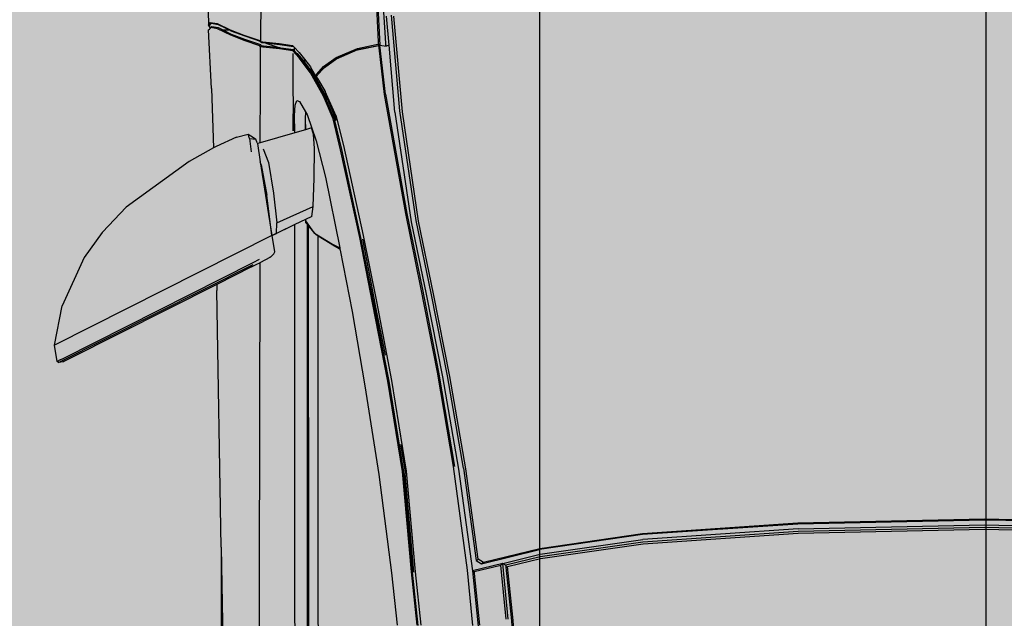
# Model space of a CAD drawing. Units: inches. Extents: x 1884 to 2398, y 474 to 1488.
# Tile 11 of 39: x 2186 to 2231, y 672 to 699. Entities that reach past the tile are written whole.
import ezdxf

# ---------------------------------------------------------------- set-up
doc = ezdxf.new("R2010")
doc.units = ezdxf.units.IN
doc.header["$MEASUREMENT"] = 0
doc.layers.get('0').update_dxf_attribs({"color": 250})
doc.layers.add('A-ANNO-DIMS', color=2, linetype='Continuous', lineweight=18)
doc.layers.add('C-VEHI', color=8, linetype='Continuous', lineweight=18)
doc.layers.add('Edges', color=250, linetype='Continuous')
doc.layers.add('L-PVMT-PATT', color=9, linetype='Continuous', lineweight=13, true_color=0xc7c8ca)
doc.styles.get("Standard").update_dxf_attribs({"font": 'arial.ttf'})
doc.dimstyles.get("Standard").update_dxf_attribs({"dimtxt": 7, "dimasz": 0.18, "dimexe": 0.18, "dimexo": 0.0625, "dimgap": 0.09, "dimtad": 0, "dimtih": 1, "dimtoh": 1, "dimzin": 0, "dimdsep": 46, "dimlunit": 3, "dimtxsty": 'Standard', "dimcen": 0.09, "dimadec": 0, "dimazin": 0, "dimtfac": 1, "dimtofl": 0, "dimtmove": 0, "dimatfit": 3, "dimfxl": 1, "dimtolj": 1, "dimtzin": 0, "dimarcsym": 0})

# ---------------------------------------------------------------- blocks, each defined once
blk = doc.blocks.new('Nissan Qashqai pl')
at = {"layer": 'Edges'}
for p, q in [((9.2241, 12.1376), (9.2195, 11.9221)), ((9.2249, 12.1376), (9.2203, 11.9221)), ((9.2259, 11.9221), (9.2305, 12.1375)), ((9.2335, 12.1374), (9.2289, 11.9221)), ((9.2308, 11.9221), (9.2355, 12.1374)), ((9.2195, 11.9221), (9.2241, 11.7066)), ((9.2203, 11.9221), (9.2249, 11.7065)), ((9.2305, 11.7067), (9.2259, 11.9221)), ((9.2289, 11.9221), (9.2335, 11.7067)), ((9.2355, 11.7068), (9.2308, 11.9221)), ((9.2241, 11.7066), (9.2362, 11.5274)), ((9.2249, 11.7065), (9.2371, 11.5273)), ((9.2305, 11.7067), (9.2426, 11.5277)), ((9.2335, 11.7067), (9.2457, 11.5277)), ((9.2476, 11.5278), (9.2355, 11.7068)), ((9.2362, 11.5274), (9.2535, 11.4087)), ((9.2371, 11.5273), (9.2543, 11.4085)), ((9.2598, 11.4093), (9.2426, 11.5277)), ((9.2457, 11.5277), (9.2629, 11.4092)), ((9.2649, 11.4094), (9.2476, 11.5278)), ((9.2535, 11.4087), (9.2694, 11.3436)), ((9.2707, 11.3414), (9.2543, 11.4085)), ((9.2704, 11.3659), (9.2598, 11.4093)), ((9.2629, 11.4092), (9.2726, 11.3695)), ((9.2741, 11.3716), (9.2649, 11.4094)), ((9.3326, 11.3776), (9.2741, 11.3716)), ((9.2746, 11.3697), (9.333, 11.3757)), ((9.4, 11.3832), (9.3326, 11.3776)), ((9.333, 11.3757), (9.4004, 11.3813)), ((9.3346, 11.3724), (9.2704, 11.3659)), ((9.2704, 11.3659), (9.2726, 11.3695)), ((9.2704, 11.3659), (9.2724, 11.3637)), ((9.2704, 11.3659), (9.2789, 11.331)), ((9.3346, 11.37), (9.2724, 11.3637)), ((9.2799, 11.3328), (9.2724, 11.3637)), ((9.2726, 11.3695), (9.2746, 11.3697)), ((9.2694, 11.3436), (9.2656, 11.3376)), ((9.2669, 11.3354), (9.2707, 11.3414)), ((9.2694, 11.3436), (9.2707, 11.3414)), ((9.2819, 11.333), (9.3418, 11.3391)), ((9.1605, 11.3208), (9.2669, 11.3354)), ((9.2656, 11.3376), (9.1612, 11.3233)), ((9.1617, 11.315), (9.2789, 11.331)), ((9.2669, 11.3354), (9.2656, 11.3376)), ((9.3422, 11.3316), (9.2783, 11.3251)), ((9.2789, 11.331), (9.3427, 11.3375)), ((9.2789, 11.331), (9.2799, 11.3327)), ((9.2799, 11.3328), (9.2819, 11.333)), ((9.2799, 11.3327), (9.2799, 11.3328)), ((9.2799, 11.3327), (9.2811, 11.3325)), ((9.1605, 11.3208), (9.0538, 11.3023)), ((9.1612, 11.3233), (9.0546, 11.3048)), ((9.2783, 11.3251), (9.1584, 11.3091)), ((9.0546, 11.3048), (8.9591, 11.2859)), ((9.1584, 11.3091), (9.0495, 11.2906)), ((9.0497, 11.2918), (9.1586, 11.3104)), ((9.0552, 11.2965), (9.1617, 11.315)), ((9.0538, 11.3023), (8.9583, 11.2833)), ((8.9598, 11.2775), (9.0552, 11.2965)), ((8.9583, 11.2833), (8.8745, 11.266)), ((8.9591, 11.2859), (8.8754, 11.2687)), ((9.0495, 11.2906), (8.9521, 11.2715)), ((8.9522, 11.2728), (9.0497, 11.2918)), ((8.8666, 11.2554), (8.9522, 11.2728)), ((8.9521, 11.2715), (8.8666, 11.2541)), ((8.8761, 11.2602), (8.9598, 11.2775)), ((9.2801, 11.2648), (9.3418, 11.2713)), ((8.8745, 11.266), (8.7481, 11.2473)), ((8.8754, 11.2687), (8.7491, 11.2501)), ((8.7496, 11.2416), (8.8761, 11.2602)), ((9.1639, 11.2546), (9.2801, 11.2648)), ((9.2803, 11.2606), (9.1644, 11.2503)), ((9.2804, 11.262), (9.1645, 11.2518)), ((9.2804, 11.2635), (9.1668, 11.2533)), ((9.3418, 11.2671), (9.2803, 11.2606)), ((9.3419, 11.2685), (9.2804, 11.262)), ((8.7491, 11.2501), (8.6386, 11.2404)), ((8.7287, 11.2307), (8.8666, 11.2554)), ((8.8666, 11.2541), (8.7292, 11.2295)), ((9.0591, 11.2377), (9.1639, 11.2546)), ((9.1644, 11.2503), (9.06, 11.2335)), ((9.1645, 11.2518), (9.0601, 11.235)), ((9.133, 11.2481), (9.1647, 11.2532)), ((9.1647, 11.2532), (9.1668, 11.2533)), ((8.7481, 11.2473), (8.6375, 11.2376)), ((8.7496, 11.2416), (8.6721, 11.2348)), ((8.9679, 11.2201), (9.0591, 11.2377)), ((9.1676, 11.2229), (9.2814, 11.2377)), ((9.2814, 11.2377), (9.3416, 11.2442)), ((8.6699, 11.231), (8.622, 11.228)), ((8.6721, 11.2348), (8.6387, 11.2319)), ((8.6721, 11.2312), (8.6699, 11.231)), ((8.6721, 11.2348), (8.6733, 11.2313)), ((8.6721, 11.2312), (8.6721, 11.2318)), ((8.6721, 11.2241), (8.6733, 11.2313)), ((8.6733, 11.2313), (8.6721, 11.2312)), ((8.7287, 11.2307), (8.6721, 11.2241)), ((8.7292, 11.2295), (8.6753, 11.2232)), ((9.0601, 11.235), (8.8941, 11.2023)), ((9.06, 11.2335), (8.9696, 11.2157)), ((8.9708, 11.2185), (9.03, 11.2304)), ((8.6683, 11.2226), (8.6197, 11.2201)), ((8.6203, 11.2213), (8.6721, 11.2241)), ((8.671, 11.2227), (8.6683, 11.2226)), ((8.6721, 11.2241), (8.671, 11.2227)), ((8.6716, 11.2199), (8.671, 11.2227)), ((8.6759, 11.1982), (8.6716, 11.2199)), ((8.6721, 11.2241), (8.6727, 11.2229)), ((8.6772, 11.1988), (8.6721, 11.2241)), ((8.6753, 11.2232), (8.6727, 11.2229)), ((8.6777, 11.1984), (8.6727, 11.2229)), ((8.8918, 11.205), (8.9679, 11.2201)), ((8.9696, 11.2157), (8.8942, 11.2009)), ((8.9318, 11.211), (8.9704, 11.2185)), ((8.9704, 11.2185), (8.9708, 11.2185)), ((9.0656, 11.207), (9.1676, 11.2229)), ((8.7881, 11.1821), (8.8918, 11.205)), ((8.8941, 11.2023), (8.7925, 11.1802)), ((8.8961, 11.204), (8.9318, 11.211)), ((8.9797, 11.1924), (9.0656, 11.207)), ((8.6864, 11.1736), (8.6759, 11.1982)), ((8.6875, 11.1744), (8.6772, 11.1988)), ((8.6777, 11.1984), (8.6883, 11.1737)), ((8.8942, 11.2009), (8.7931, 11.1789)), ((8.9087, 11.1783), (8.9797, 11.1924)), ((8.7575, 11.1744), (8.7881, 11.1821)), ((8.7925, 11.1802), (8.7591, 11.1723)), ((8.697, 11.1592), (8.6864, 11.1736)), ((8.6979, 11.1603), (8.6875, 11.1744)), ((8.6883, 11.1737), (8.6987, 11.1597)), ((8.7508, 11.1722), (8.7257, 11.1609)), ((8.7529, 11.17), (8.7302, 11.1602)), ((8.7574, 11.1704), (8.7312, 11.1591)), ((8.7346, 11.1636), (8.7577, 11.1732)), ((8.7346, 11.1636), (8.7491, 11.1703)), ((8.7491, 11.1703), (8.7576, 11.1743)), ((8.7508, 11.1722), (8.7491, 11.1703)), ((8.7532, 11.1733), (8.7508, 11.1722)), ((8.7529, 11.17), (8.7577, 11.1732)), ((8.757, 11.1718), (8.7529, 11.17)), ((8.7532, 11.1733), (8.7575, 11.1744)), ((8.7587, 11.1722), (8.757, 11.1718)), ((8.7931, 11.1789), (8.7574, 11.1704)), ((8.7575, 11.1744), (8.7576, 11.1743)), ((8.7576, 11.1743), (8.7582, 11.1734)), ((8.7577, 11.1732), (8.7582, 11.1734)), ((8.7582, 11.1734), (8.759, 11.1725)), ((8.759, 11.1725), (8.7587, 11.1722)), ((8.7591, 11.1723), (8.7587, 11.1722)), ((8.759, 11.1725), (8.7591, 11.1723)), ((8.8245, 11.1613), (8.9063, 11.1779)), ((8.8893, 11.1486), (8.9021, 11.1697)), ((8.9041, 11.1717), (8.8927, 11.1528)), ((8.9021, 11.1697), (8.9063, 11.1779)), ((8.9075, 11.1781), (8.9041, 11.1717)), ((8.9063, 11.1779), (8.9075, 11.1781)), ((8.9075, 11.1781), (8.9087, 11.1783)), ((8.7055, 11.1514), (8.697, 11.1592)), ((8.6987, 11.1596), (8.6979, 11.1603)), ((8.6987, 11.1597), (8.6988, 11.1596)), ((8.6987, 11.1596), (8.6988, 11.1596)), ((8.6996, 11.1588), (8.6987, 11.1596)), ((8.6988, 11.1596), (8.6996, 11.1588)), ((8.6996, 11.1588), (8.6996, 11.1588)), ((8.7062, 11.1527), (8.6996, 11.1588)), ((8.6996, 11.1588), (8.7062, 11.1527)), ((8.7302, 11.1602), (8.7032, 11.145)), ((8.7312, 11.1591), (8.7042, 11.144)), ((8.7075, 11.1487), (8.7346, 11.1636)), ((8.7108, 11.1523), (8.7257, 11.1609)), ((8.7108, 11.1523), (8.7248, 11.1605)), ((8.7248, 11.1605), (8.7257, 11.1609)), ((8.7828, 11.1508), (8.8245, 11.1613)), ((8.6917, 11.1371), (8.7075, 11.1487)), ((8.7071, 11.15), (8.6981, 11.1446)), ((8.707, 11.15), (8.7055, 11.1514)), ((8.7067, 11.1522), (8.7062, 11.1527)), ((8.7083, 11.1508), (8.7067, 11.1522)), ((8.707, 11.15), (8.7083, 11.1508)), ((8.7071, 11.15), (8.707, 11.15)), ((8.707, 11.15), (8.707, 11.15)), ((8.7083, 11.1508), (8.7071, 11.15)), ((8.7083, 11.1507), (8.7102, 11.1519)), ((8.7083, 11.1508), (8.7083, 11.1507)), ((8.7102, 11.1519), (8.7108, 11.1523)), ((8.7524, 11.1401), (8.7828, 11.1508)), ((8.7748, 11.1475), (8.7678, 11.1453)), ((8.7678, 11.1453), (8.7698, 11.1385)), ((8.7916, 11.1488), (8.7748, 11.1475)), ((8.8259, 11.1483), (8.7916, 11.1488)), ((8.8585, 11.1473), (8.8259, 11.1483)), ((8.87, 11.1455), (8.8585, 11.1473)), ((8.8771, 11.1054), (8.8585, 11.1473)), ((8.87, 11.1455), (8.8734, 11.1385)), ((8.8893, 11.1486), (8.8751, 11.1387)), ((8.881, 11.1418), (8.8893, 11.1486)), ((8.8913, 11.1506), (8.8893, 11.1486)), ((8.8927, 11.1528), (8.8913, 11.1506)), ((9.3225, 11.1531), (8.8927, 11.1528)), ((9.4936, 11.1538), (9.3225, 11.1531)), ((8.6805, 11.1309), (8.6884, 11.1371)), ((8.6818, 11.1288), (8.6902, 11.136)), ((8.6927, 11.1371), (8.6859, 11.132)), ((8.7042, 11.144), (8.687, 11.131)), ((8.6884, 11.1371), (8.6973, 11.144)), ((8.6884, 11.1371), (8.6917, 11.1371)), ((8.6902, 11.136), (8.6917, 11.1371)), ((8.6923, 11.1371), (8.6927, 11.1371)), ((8.7032, 11.145), (8.6927, 11.1371)), ((8.6973, 11.144), (8.698, 11.1446)), ((8.698, 11.1446), (8.6981, 11.1446)), ((8.7373, 11.1314), (8.7492, 11.1383)), ((8.7492, 11.1383), (8.7524, 11.1401)), ((8.7492, 11.1383), (8.7572, 11.1379)), ((8.7572, 11.1379), (8.7698, 11.1383)), ((8.7698, 11.1385), (8.7583, 11.1382)), ((8.7698, 11.1385), (8.7698, 11.1383)), ((8.7698, 11.1383), (8.7733, 11.126)), ((8.8734, 11.1385), (8.8793, 11.1261)), ((8.8734, 11.1385), (8.8768, 11.1385)), ((8.8751, 11.1387), (8.8768, 11.1385)), ((8.8768, 11.1385), (8.879, 11.1402)), ((8.879, 11.1402), (8.881, 11.1418)), ((8.879, 11.1402), (9.3198, 11.1403)), ((9.3225, 11.1421), (8.881, 11.1418)), ((9.3198, 11.1403), (9.4922, 11.1409)), ((9.4936, 11.1428), (9.3225, 11.1421)), ((8.6703, 11.1081), (8.6727, 11.1235)), ((8.6714, 11.1088), (8.6737, 11.1245)), ((8.6727, 11.1235), (8.6737, 11.1245)), ((8.6737, 11.1245), (8.6746, 11.1253)), ((8.6805, 11.1309), (8.6746, 11.1253)), ((8.6746, 11.1253), (8.6785, 11.1253)), ((8.6777, 11.1246), (8.6755, 11.1099)), ((8.6788, 11.1237), (8.6764, 11.1083)), ((8.6785, 11.1253), (8.6777, 11.1246)), ((8.6815, 11.128), (8.6785, 11.1253)), ((8.687, 11.131), (8.6788, 11.1237)), ((8.6815, 11.128), (8.6818, 11.1288)), ((8.6817, 11.1282), (8.6815, 11.128)), ((8.6859, 11.132), (8.6817, 11.1282)), ((8.6817, 11.1282), (8.6818, 11.1288)), ((8.6818, 11.1238), (8.7026, 11.1238)), ((8.7026, 11.1238), (8.7026, 11.1239)), ((8.7026, 11.1238), (8.7072, 11.1239)), ((8.7072, 11.1239), (8.7072, 11.1239)), ((8.7072, 11.1239), (8.7273, 11.1239)), ((8.7273, 11.1239), (8.7273, 11.124)), ((8.7273, 11.1239), (8.7354, 11.124)), ((8.7354, 11.1241), (8.7354, 11.124)), ((8.7354, 11.124), (8.742, 11.124)), ((8.7361, 11.1283), (8.7373, 11.1314)), ((8.7415, 11.1265), (8.7361, 11.1283)), ((8.7534, 11.1257), (8.7415, 11.1265)), ((8.742, 11.1241), (8.742, 11.124)), ((8.742, 11.124), (8.742, 11.1241)), ((8.742, 11.124), (8.742, 11.124)), ((8.742, 11.124), (8.7426, 11.124)), ((8.7426, 11.1241), (8.7426, 11.124)), ((8.7426, 11.124), (8.7433, 11.124)), ((8.7433, 11.1241), (8.7433, 11.124)), ((8.7433, 11.124), (8.7711, 11.1241)), ((8.7711, 11.1241), (8.7516, 11.1241)), ((8.7718, 11.126), (8.7534, 11.1257)), ((8.7733, 11.126), (8.7718, 11.126)), ((8.7733, 11.126), (8.7849, 11.0859)), ((9.3194, 11.1262), (8.8793, 11.1261)), ((8.8793, 11.1261), (8.8815, 11.1214)), ((9.4919, 11.1269), (9.3194, 11.1262)), ((8.8815, 11.1214), (8.892, 11.0998)), ((8.8815, 11.1214), (8.8895, 11.1048)), ((8.6684, 11.0892), (8.6703, 11.1081)), ((8.6697, 11.0922), (8.6714, 11.1088)), ((8.6698, 11.0925), (8.6755, 11.1099)), ((8.6754, 11.1089), (8.6735, 11.0898)), ((8.6764, 11.1082), (8.6744, 11.0891)), ((8.6755, 11.1099), (8.6754, 11.1089)), ((8.6764, 11.1082), (8.6764, 11.1083)), ((8.807, 11.0862), (8.8918, 11.0997)), ((8.8075, 11.0955), (8.8429, 11.1016)), ((8.8429, 11.1016), (8.8771, 11.1054)), ((8.8918, 11.0997), (8.8455, 11.0936)), ((8.8895, 11.1048), (8.8771, 11.1054)), ((8.8908, 11.1021), (8.8895, 11.1048)), ((8.8906, 11.1024), (8.8895, 11.1048)), ((8.8906, 11.1024), (8.8911, 11.1013)), ((8.892, 11.0998), (8.8908, 11.1021)), ((8.8911, 11.1013), (8.8919, 11.0997)), ((8.8911, 11.1013), (8.8919, 11.0998)), ((8.8919, 11.0997), (8.8911, 11.1013)), ((8.8919, 11.0997), (8.8918, 11.0997)), ((8.8918, 11.0997), (9.0186, 10.8486)), ((8.892, 11.0998), (8.8919, 11.0998)), ((8.8919, 11.0998), (8.8919, 11.0997)), ((8.8919, 11.0997), (8.8919, 11.0997)), ((8.9106, 11.1029), (8.892, 11.0998)), ((8.892, 11.0998), (8.892, 11.0998)), ((8.9131, 11.102), (8.9106, 11.1029)), ((8.9171, 11.0978), (8.9131, 11.102)), ((8.6682, 11.087), (8.6684, 11.0888)), ((8.6684, 11.0888), (8.6684, 11.0892)), ((8.6684, 11.0888), (8.6685, 11.089)), ((8.6692, 11.0876), (8.6697, 11.0922)), ((8.6697, 11.0922), (8.6698, 11.0925)), ((8.6735, 11.0898), (8.6733, 11.0875)), ((8.6744, 11.0891), (8.6742, 11.0866)), ((8.7917, 11.0895), (8.8075, 11.0955)), ((8.8102, 11.0874), (8.8455, 11.0936)), ((8.9171, 11.0978), (8.917, 11.0974)), ((8.9171, 11.0978), (8.9233, 11.0855)), ((8.5326, 11.0874), (8.6675, 11.0866)), ((8.6606, 11.0674), (8.6667, 11.0857)), ((8.6616, 11.0683), (8.6675, 11.0862)), ((8.6718, 11.0868), (8.6657, 11.0684)), ((8.6667, 11.0857), (8.6675, 11.0862)), ((8.6728, 11.0858), (8.6667, 11.0675)), ((8.6674, 11.0864), (8.6675, 11.0865)), ((8.6675, 11.0865), (8.6675, 11.0866)), ((8.6676, 11.0866), (8.6675, 11.0866)), ((8.6675, 11.0862), (8.6679, 11.0864)), ((8.6676, 11.0864), (8.6677, 11.0866)), ((8.6677, 11.0866), (8.6676, 11.0866)), ((8.6682, 11.0866), (8.6677, 11.0866)), ((8.6679, 11.0864), (8.6682, 11.0866)), ((8.6692, 11.0876), (8.6682, 11.0866)), ((8.6682, 11.087), (8.6692, 11.0876)), ((8.6682, 11.0866), (8.6682, 11.087)), ((8.6729, 11.0874), (8.6718, 11.0868)), ((8.674, 11.0864), (8.6728, 11.0858)), ((8.6733, 11.0875), (8.6729, 11.0874)), ((8.6742, 11.0866), (8.674, 11.0864)), ((8.6744, 11.0866), (8.6742, 11.0866)), ((8.6742, 11.0858), (8.6743, 11.086)), ((8.6744, 11.0864), (8.6744, 11.0866)), ((8.6773, 11.0865), (8.6744, 11.0866)), ((8.6791, 11.0864), (8.677, 11.0864)), ((8.6791, 11.0865), (8.6773, 11.0865)), ((8.6791, 11.0865), (8.6791, 11.0864)), ((8.6878, 11.0864), (8.6791, 11.0865)), ((8.7205, 11.0863), (8.6791, 11.0864)), ((8.6878, 11.0864), (8.6791, 11.0864)), ((8.6878, 11.0865), (8.6878, 11.0864)), ((8.6911, 11.0864), (8.6878, 11.0864)), ((8.7205, 11.0863), (8.6911, 11.0864)), ((8.7849, 11.0859), (8.7205, 11.0863)), ((8.7751, 11.0723), (8.7779, 11.0773)), ((8.7779, 11.0773), (8.7807, 11.0812)), ((8.7798, 11.0739), (8.7807, 11.0812)), ((8.7849, 11.0827), (8.7807, 11.0812)), ((8.7849, 11.0859), (8.7856, 11.0834)), ((8.7849, 11.0827), (8.7858, 11.0828)), ((8.7858, 11.0828), (8.7856, 11.0834)), ((8.7858, 11.0828), (8.807, 11.0862)), ((8.8102, 11.0874), (8.807, 11.0862)), ((8.9232, 11.0779), (8.9194, 11.0854)), ((9.0333, 10.8597), (8.9232, 11.0779)), ((8.9233, 11.0855), (9.2886, 11.0848)), ((8.925, 11.0821), (8.9233, 11.0855)), ((8.928, 11.0762), (8.925, 11.0821)), ((9.0386, 10.8534), (8.9254, 11.0778)), ((9.2886, 11.0848), (9.4673, 11.0852)), ((8.6546, 11.0516), (8.6606, 11.0674)), ((8.6556, 11.0524), (8.6616, 11.0683)), ((8.6657, 11.0684), (8.6598, 11.0529)), ((8.6667, 11.0675), (8.6608, 11.0521)), ((8.7798, 11.0739), (8.7751, 11.0723)), ((8.7785, 11.0587), (8.7751, 11.0723)), ((8.7798, 11.0739), (8.7954, 11.0758)), ((8.928, 11.0762), (8.9483, 11.0359)), ((8.7785, 11.0587), (8.7891, 11.0353)), ((8.6472, 11.0366), (8.6546, 11.0516)), ((8.6482, 11.0375), (8.655, 11.0513)), ((8.655, 11.0432), (8.6524, 11.0378)), ((8.6608, 11.0521), (8.6534, 11.0369)), ((8.6598, 11.0529), (8.655, 11.0432)), ((8.655, 11.0513), (8.6556, 11.0524)), ((8.655, 11.0513), (8.655, 11.0432)), ((9.2517, 11.0411), (9.5372, 11.0459)), ((8.646, 11.0289), (8.6468, 11.0337)), ((8.6468, 11.0337), (8.6472, 11.0366)), ((8.647, 11.03), (8.6468, 11.0337)), ((8.647, 11.03), (8.6482, 11.0375)), ((8.6524, 11.0378), (8.651, 11.0302)), ((8.6534, 11.0369), (8.652, 11.0292)), ((8.7222, 11.0298), (8.7908, 11.0322)), ((8.7891, 11.0353), (8.7908, 11.0322)), ((8.7908, 11.0322), (8.8066, 11.0041)), ((8.9483, 11.0359), (8.9552, 11.0361)), ((8.9483, 11.0359), (9.0343, 10.8656)), ((9.2517, 11.0411), (8.9552, 11.0361)), ((9.2517, 11.0411), (9.351, 11.0411)), ((8.5838, 11.0251), (8.6489, 11.0263)), ((8.6489, 11.0263), (8.646, 11.0289)), ((8.6498, 11.0273), (8.647, 11.03)), ((8.6527, 11.0286), (8.6489, 11.0263)), ((8.6524, 11.0289), (8.6498, 11.0273)), ((8.651, 11.0302), (8.652, 11.0292)), ((8.652, 11.0292), (8.6524, 11.0289)), ((8.6524, 11.0289), (8.6527, 11.0286)), ((8.6527, 11.0286), (8.6537, 11.0275)), ((8.6547, 11.0265), (8.6537, 11.0275)), ((8.6537, 11.0275), (8.6537, 11.0275)), ((8.7222, 11.0298), (8.6547, 11.0265)), ((8.8066, 11.0041), (8.8591, 10.9315)), ((8.8591, 10.9315), (8.8879, 10.9041)), ((8.8885, 10.9037), (8.8879, 10.9041)), ((8.8885, 10.9037), (8.9173, 10.8831)), ((8.9173, 10.8831), (8.9731, 10.8577)), ((9.0343, 10.8656), (9.0347, 10.8648)), ((9.0347, 10.8648), (9.0362, 10.8619)), ((9.0362, 10.8619), (9.037, 10.8603)), ((9.0186, 10.8486), (8.9731, 10.8577)), ((9.0374, 10.8517), (9.0186, 10.8486)), ((9.0356, 10.8553), (9.0333, 10.8597)), ((9.0356, 10.8553), (9.0374, 10.8517)), ((9.0371, 10.8601), (9.037, 10.8603)), ((9.0371, 10.8601), (9.0376, 10.8591)), ((9.0376, 10.8591), (9.0371, 10.8595)), ((9.0386, 10.8534), (9.0374, 10.8517)), ((9.0376, 10.8591), (9.0386, 10.8534))]:
    blk.add_line(p, q, dxfattribs=at)
blk = doc.blocks.new('car')
blk.add_blockref('Nissan Qashqai pl', (-9.7433, -11.9151))
blk = doc.blocks.new('carr')
blk.add_blockref('car', (0.5124, -0.007))
blk = doc.blocks.new('*D44')
at = {"layer": 'A-ANNO-DIMS', "color": 0, "lineweight": -2, "transparency": 16777216}
for p, q in [((2209.755, 1247.822), (2209.755, 484.005)), ((2230.029, 1247.822), (2230.029, 484.005)), ((2209.935, 484.185), (2229.849, 484.185)), ((2230.029, 484.185), (2230.209, 484.185))]:
    blk.add_line(p, q, dxfattribs=at)
at = {"layer": 'A-ANNO-DIMS', "color": 0, "lineweight": 100, "transparency": 16777216}
for points in [[(2209.935, 484.215), (2209.935, 484.155), (2209.755, 484.185)], [(2229.849, 484.215), (2229.849, 484.155), (2230.029, 484.185)]]:
    blk.add_solid(points, dxfattribs=at)
at = {"layer": 'Defpoints', "color": 0, "lineweight": 100, "transparency": 16777216}
for p in [(2209.755, 1247.885), (2230.029, 1247.885), (2230.029, 484.185)]:
    blk.add_point(p, dxfattribs=at)
at = {"layer": 'A-ANNO-DIMS', "color": 0, "transparency": 16777216, "insert": (2247.429, 484.185), "char_height": 7, "attachment_point": 5}
blk.add_mtext('\\A1;1\'-8 1/2"', dxfattribs=at)

msp = doc.modelspace()

# ---------------------------------------------------------------- hatches: boundary and pattern name
at = {"layer": 'L-PVMT-PATT'}
h = msp.add_hatch(color=256, dxfattribs=at)
h.dxf.hatch_style = 1
h.paths.add_polyline_path([(2387.529, 769.966), (2351.529, 769.966), (2238.447, 769.966), (2238.447, 762.15), (2238.447, 754.445), (2126.529, 754.445), (2126.529, 676.183), (2134.868, 676.183), (2142.673, 676.183), (2142.673, 646.578), (2134.868, 646.578), (2126.529, 646.578), (2126.529, 640.17), (2387.529, 640.17)])
h.paths.add_polyline_path([(2387.529, 631.385), (2303.086, 631.385), (2303.086, 615.671), (2387.529, 615.671)])
h.paths.add_polyline_path([(2387.529, 640.17), (2126.529, 640.17), (2126.529, 631.385), (2387.529, 631.385)])
h.paths.add_polyline_path([(2393.529, 604.13), (2387.529, 604.13), (2387.529, 615.671), (2303.086, 615.671), (2303.086, 607.943), (2249.649, 607.943), (2126.529, 607.943), (2126.529, 533.885), (2393.529, 533.885)])
h.paths.add_polyline_path([(2257.825, 611.008), (2257.83, 611.337), (2257.915, 616.493), (2258.021, 621.805), (2258.146, 627.274), (2258.252, 631.385), (2126.529, 631.385), (2126.529, 611.008)])
h.paths.add_polyline_path([(2258.892, 611.285), (2258.888, 611.008), (2300.247, 611.008), (2300.247, 631.385), (2259.314, 631.385), (2259.206, 627.173), (2259.081, 621.72), (2258.976, 616.424)])

# ---------------------------------------------------------------- block references
at = {"layer": 'C-VEHI', "xscale": 39.37007874015748, "yscale": 39.37007874015748, "zscale": 39.37007874015748, "rotation": 270}
msp.add_blockref('carr', (2229.977, 676.232), dxfattribs=at)

# ---------------------------------------------------------------- dimensions: what is measured, and where the dimension line sits
at = {"layer": 'A-ANNO-DIMS'}
dim = msp.add_linear_dim(base=(2230.029, 484.185), p1=(2209.755, 1247.885), p2=(2230.029, 1247.885), dimstyle='Standard', override={"dimdec": 1, "dimlfac": 1, "dimrnd": 0, "dimzin": 1, "dimdsep": 46, "dimlunit": 4, "dimfrac": 2}, dxfattribs=at)
dim.commit()
dim.dimension.update_dxf_attribs({"geometry": '*D44', "text_midpoint": (2247.429, 484.185)})

doc.saveas('drawing.dxf')
